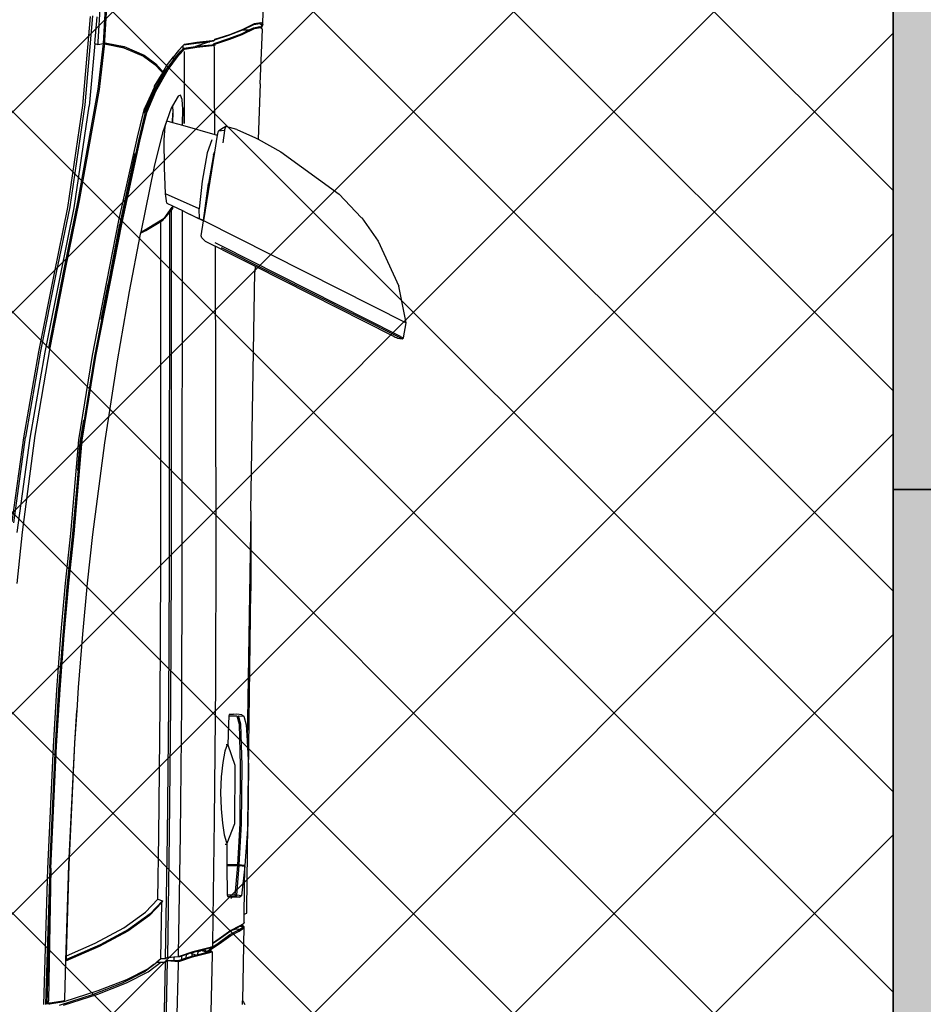
# Model space of a CAD drawing. Units: inches. Extents: x 2167 to 2589, y 1680 to 2489.
# Tile 19 of 38: x 2387 to 2419, y 1761 to 1796. Entities that reach past the tile are written whole.
import ezdxf

# ---------------------------------------------------------------- set-up
doc = ezdxf.new("R2010")
doc.units = ezdxf.units.IN
doc.header["$MEASUREMENT"] = 0
doc.layers.get('0').update_dxf_attribs({"color": 250})
doc.layers.add('A-FLOR-PATT', color=254, linetype='Continuous', lineweight=13, true_color=0xfeeab9)
for name, color, linetype, lineweight in [('A-WALL-PATT', 250, 'Continuous', 13), ('C-PRKG-VEHS', 8, 'Continuous', 13), ('L-PVMT-PATT', 252, 'Continuous', 13), ('walls', 7, 'Continuous', 35)]:
    doc.layers.add(name, color=color, linetype=linetype, lineweight=lineweight)
doc.layers.add('Edges', color=250, linetype='Continuous')

# ---------------------------------------------------------------- blocks, each defined once
blk = doc.blocks.new('Nissan Qashqai pl')
at = {"layer": 'Edges'}
for p, q in [((8.8918, 12.7444), (9.0186, 12.9956)), ((9.0386, 12.9907), (8.9254, 12.7664)), ((9.0186, 12.9956), (8.9731, 12.9865)), ((9.0374, 12.9925), (9.0186, 12.9956)), ((9.0356, 12.9888), (9.0333, 12.9845)), ((9.0356, 12.9888), (9.0374, 12.9925)), ((9.0386, 12.9907), (9.0374, 12.9925)), ((9.0376, 12.985), (9.0386, 12.9907)), ((8.9173, 12.961), (8.9731, 12.9865)), ((9.0333, 12.9845), (8.9232, 12.7662)), ((8.9483, 12.8082), (9.0343, 12.9785)), ((9.0343, 12.9785), (9.0347, 12.9794)), ((9.0347, 12.9794), (9.0362, 12.9822)), ((9.0362, 12.9822), (9.037, 12.9838)), ((9.0371, 12.9841), (9.037, 12.9838)), ((9.0371, 12.9841), (9.0376, 12.985)), ((9.0376, 12.985), (9.0371, 12.9847)), ((8.8885, 12.9405), (8.9173, 12.961)), ((8.8591, 12.9127), (8.8879, 12.94)), ((8.8885, 12.9405), (8.8879, 12.94)), ((8.8066, 12.84), (8.8591, 12.9127)), ((8.7908, 12.812), (8.8066, 12.84)), ((8.6489, 12.8179), (8.5719, 12.8193)), ((8.646, 12.8153), (8.6489, 12.8179)), ((8.6489, 12.8179), (8.6527, 12.8156)), ((8.6547, 12.8176), (8.6537, 12.8167)), ((8.7222, 12.8144), (8.6547, 12.8176)), ((8.646, 12.8153), (8.646, 12.8153)), ((8.6472, 12.8076), (8.646, 12.8153)), ((8.647, 12.8142), (8.6498, 12.8168)), ((8.6482, 12.8067), (8.647, 12.8142)), ((8.6546, 12.7926), (8.6472, 12.8076)), ((8.655, 12.7929), (8.6482, 12.8067)), ((8.6498, 12.8168), (8.6524, 12.8153)), ((8.651, 12.814), (8.652, 12.815)), ((8.6524, 12.8064), (8.651, 12.814)), ((8.652, 12.815), (8.6524, 12.8153)), ((8.6534, 12.8073), (8.652, 12.815)), ((8.6524, 12.8153), (8.6527, 12.8156)), ((8.655, 12.801), (8.6524, 12.8064)), ((8.6527, 12.8156), (8.6537, 12.8167)), ((8.6608, 12.7921), (8.6534, 12.8073)), ((8.6537, 12.8167), (8.6537, 12.8166)), ((8.7222, 12.8144), (8.7908, 12.812)), ((8.7785, 12.7855), (8.7891, 12.8089)), ((8.7891, 12.8089), (8.7908, 12.812)), ((8.928, 12.7679), (8.9483, 12.8082)), ((8.9483, 12.8082), (8.9552, 12.8081)), ((9.2517, 12.8031), (8.9552, 12.8081)), ((8.6606, 12.7768), (8.6546, 12.7926)), ((8.6598, 12.7913), (8.655, 12.801)), ((8.655, 12.7929), (8.655, 12.801)), ((8.6556, 12.7918), (8.655, 12.7929)), ((8.655, 12.7922), (8.655, 12.7929)), ((9.2517, 12.8031), (9.351, 12.803)), ((9.2517, 12.8031), (9.5372, 12.7983)), ((9.641, 12.7991), (9.351, 12.803)), ((9.5052, 12.7918), (9.5069, 12.7941)), ((9.5061, 12.7878), (9.5069, 12.7941)), ((9.5069, 12.7941), (9.5176, 12.7972)), ((9.5176, 12.7972), (9.5372, 12.7983)), ((9.5372, 12.7983), (9.5689, 12.7999)), ((9.5689, 12.7999), (9.641, 12.7991)), ((9.641, 12.7991), (9.6921, 12.7956)), ((9.7466, 12.7978), (9.641, 12.7991)), ((9.692, 12.7943), (9.6913, 12.7886)), ((9.6921, 12.7956), (9.692, 12.7943)), ((9.6922, 12.7943), (9.692, 12.7943)), ((9.6922, 12.7943), (9.6921, 12.7956)), ((9.7526, 12.7946), (9.6921, 12.7956)), ((9.6922, 12.7885), (9.693, 12.7955)), ((9.6922, 12.7885), (9.6922, 12.7943)), ((9.693, 12.7955), (9.7296, 12.7914)), ((9.7511, 12.7979), (9.7466, 12.7978)), ((9.7526, 12.7946), (9.7511, 12.7979)), ((9.7623, 12.7945), (9.7526, 12.7946)), ((9.7623, 12.7945), (9.7643, 12.7937)), ((9.7643, 12.7937), (9.7652, 12.7927)), ((9.7643, 12.7937), (9.7648, 12.7929)), ((9.7648, 12.7929), (9.7648, 12.7929)), ((9.7648, 12.7929), (9.7664, 12.7902)), ((9.7652, 12.7927), (9.7665, 12.7907)), ((9.7667, 12.7933), (9.7665, 12.7907)), ((9.7677, 12.7944), (9.7667, 12.7933)), ((9.7676, 12.7931), (9.7667, 12.7933)), ((9.7673, 12.7899), (9.7676, 12.7931)), ((9.769, 12.7926), (9.7676, 12.7931)), ((9.7677, 12.7944), (9.7677, 12.7944)), ((9.77, 12.7936), (9.7677, 12.7944)), ((9.7677, 12.7944), (9.8598, 12.7928)), ((9.7712, 12.7892), (9.769, 12.7926)), ((9.7734, 12.7884), (9.77, 12.7936)), ((9.8598, 12.7928), (9.8614, 12.7937)), ((9.8643, 12.7927), (9.8598, 12.7928)), ((9.8614, 12.7937), (9.8647, 12.7956)), ((8.6616, 12.7758), (8.6556, 12.7918)), ((8.6657, 12.7758), (8.6598, 12.7913)), ((8.6667, 12.7767), (8.6608, 12.7921)), ((8.7785, 12.7855), (8.7751, 12.7719)), ((9.5037, 12.7806), (9.5045, 12.7814)), ((9.5052, 12.7918), (9.5044, 12.7856)), ((9.5044, 12.7856), (9.5045, 12.7814)), ((9.5045, 12.7814), (9.5045, 12.7759)), ((9.5168, 12.7904), (9.5061, 12.7878)), ((9.5061, 12.7856), (9.5167, 12.7883)), ((9.5063, 12.7755), (9.5061, 12.7856)), ((9.5167, 12.7883), (9.5679, 12.7899)), ((9.5679, 12.792), (9.5168, 12.7904)), ((9.5678, 12.7837), (9.5426, 12.7747)), ((9.64, 12.7831), (9.5678, 12.7837)), ((9.6401, 12.7914), (9.5679, 12.792)), ((9.5679, 12.7899), (9.64, 12.7892)), ((9.64, 12.7892), (9.6912, 12.7865)), ((9.6645, 12.7737), (9.64, 12.7831)), ((9.6913, 12.7886), (9.6401, 12.7914)), ((9.6912, 12.7811), (9.6911, 12.7796)), ((9.6913, 12.7886), (9.6912, 12.7865)), ((9.6912, 12.7865), (9.6912, 12.7811)), ((9.692, 12.7811), (9.6912, 12.7811)), ((9.692, 12.7811), (9.6921, 12.7864)), ((9.692, 12.7796), (9.692, 12.7811)), ((9.6922, 12.7885), (9.6921, 12.7864)), ((9.6921, 12.7864), (9.7288, 12.7832)), ((9.7288, 12.7854), (9.6922, 12.7885)), ((9.7288, 12.7832), (9.7287, 12.7734)), ((9.7296, 12.7914), (9.7288, 12.7854)), ((9.7306, 12.7834), (9.7288, 12.7854)), ((9.7288, 12.7854), (9.7288, 12.7832)), ((9.7288, 12.7832), (9.7306, 12.7834)), ((9.7296, 12.7914), (9.7314, 12.7895)), ((9.7305, 12.7738), (9.7306, 12.7834)), ((9.7306, 12.7834), (9.7314, 12.7895)), ((9.7314, 12.7895), (9.7313, 12.7798)), ((9.7665, 12.7904), (9.7664, 12.7902)), ((9.7664, 12.7902), (9.7674, 12.7885)), ((9.7665, 12.7907), (9.7676, 12.7889)), ((9.7673, 12.7897), (9.7673, 12.7899)), ((9.7673, 12.7897), (9.7676, 12.7889)), ((9.7674, 12.7885), (9.7728, 12.7781)), ((9.7676, 12.7889), (9.7684, 12.7875)), ((9.7676, 12.7887), (9.7678, 12.7882)), ((9.7684, 12.7875), (9.7717, 12.781)), ((9.7707, 12.7848), (9.7709, 12.7893)), ((9.7717, 12.781), (9.7707, 12.7848)), ((9.7709, 12.7893), (9.7712, 12.7892)), ((9.7724, 12.7874), (9.7712, 12.7892)), ((9.7717, 12.781), (9.7738, 12.7771)), ((9.7778, 12.777), (9.7724, 12.7874)), ((9.7788, 12.778), (9.7734, 12.7884)), ((8.6667, 12.7584), (8.6606, 12.7768)), ((8.6675, 12.758), (8.6616, 12.7758)), ((8.6718, 12.7574), (8.6657, 12.7758)), ((8.6728, 12.7584), (8.6667, 12.7767)), ((8.7751, 12.7719), (8.7779, 12.7668)), ((8.7798, 12.7703), (8.7751, 12.7719)), ((8.7798, 12.7703), (8.7807, 12.763)), ((8.7798, 12.7703), (8.7954, 12.7683)), ((9.5045, 12.7759), (9.5063, 12.7755)), ((9.5063, 12.7755), (9.5168, 12.7751)), ((9.5168, 12.7751), (9.5423, 12.7746)), ((9.5423, 12.7746), (9.5422, 12.7736)), ((9.5422, 12.7736), (9.5422, 12.7725)), ((9.5422, 12.7736), (9.5424, 12.7735)), ((9.5426, 12.7747), (9.5423, 12.7746)), ((9.5426, 12.7747), (9.5424, 12.7735)), ((9.5424, 12.7735), (9.5503, 12.7706)), ((9.5503, 12.7706), (9.5641, 12.7681)), ((9.6395, 12.7676), (9.654, 12.7697)), ((9.654, 12.7697), (9.6633, 12.7726)), ((9.6633, 12.7726), (9.6645, 12.7737)), ((9.6655, 12.7733), (9.6645, 12.7737)), ((9.6655, 12.7733), (9.6911, 12.7732)), ((9.6655, 12.7713), (9.6655, 12.7733)), ((9.6911, 12.7796), (9.6911, 12.7732)), ((9.6911, 12.7732), (9.692, 12.7733)), ((9.692, 12.7733), (9.692, 12.7796)), ((9.692, 12.7733), (9.7287, 12.7734)), ((9.7287, 12.7734), (9.7305, 12.7738)), ((9.7305, 12.7738), (9.7313, 12.7798)), ((9.733, 12.7782), (9.7313, 12.7798)), ((9.7728, 12.7781), (9.7832, 12.7637)), ((9.7738, 12.7771), (9.7842, 12.7627)), ((9.7883, 12.7626), (9.7778, 12.777)), ((9.7894, 12.7636), (9.7788, 12.778)), ((8.6675, 12.758), (8.6667, 12.7584)), ((8.6679, 12.7578), (8.6675, 12.758)), ((8.6676, 12.7576), (8.6675, 12.7576)), ((8.6675, 12.7576), (8.6675, 12.7576)), ((8.6675, 12.7576), (8.6676, 12.7576)), ((8.6676, 12.7576), (8.6677, 12.7576)), ((8.6677, 12.7576), (8.6677, 12.7576)), ((8.6677, 12.7576), (8.6682, 12.7576)), ((8.6682, 12.7576), (8.6679, 12.7578)), ((8.6682, 12.7576), (8.6692, 12.7566)), ((8.6682, 12.7572), (8.6682, 12.7576)), ((8.6684, 12.7554), (8.6682, 12.7572)), ((8.6682, 12.7572), (8.6692, 12.7566)), ((8.6692, 12.7566), (8.6697, 12.7519)), ((8.6729, 12.7568), (8.6718, 12.7574)), ((8.674, 12.7578), (8.6728, 12.7584)), ((8.6733, 12.7566), (8.6729, 12.7568)), ((8.6735, 12.7544), (8.6733, 12.7566)), ((8.6742, 12.7576), (8.674, 12.7578)), ((8.6742, 12.7584), (8.6743, 12.7582)), ((8.6744, 12.755), (8.6742, 12.7576)), ((8.6744, 12.7576), (8.6742, 12.7576)), ((8.6744, 12.7578), (8.6744, 12.7576)), ((8.6773, 12.7577), (8.6744, 12.7576)), ((8.6791, 12.7578), (8.677, 12.7578)), ((8.6791, 12.7577), (8.6773, 12.7577)), ((8.7205, 12.7579), (8.6791, 12.7578)), ((8.6791, 12.7577), (8.6791, 12.7578)), ((8.6878, 12.7577), (8.6791, 12.7578)), ((8.6878, 12.7577), (8.6791, 12.7577)), ((8.6878, 12.7577), (8.6878, 12.7577)), ((8.6911, 12.7577), (8.6878, 12.7577)), ((8.7205, 12.7579), (8.6911, 12.7577)), ((8.7849, 12.7582), (8.7205, 12.7579)), ((8.7734, 12.7181), (8.7849, 12.7582)), ((8.7779, 12.7668), (8.7807, 12.763)), ((8.7849, 12.7615), (8.7807, 12.763)), ((8.7849, 12.7615), (8.7858, 12.7613)), ((8.7849, 12.7582), (8.7856, 12.7608)), ((8.7858, 12.7613), (8.7856, 12.7608)), ((8.7858, 12.7613), (8.807, 12.758)), ((8.8102, 12.7568), (8.807, 12.758)), ((8.807, 12.758), (8.8918, 12.7444)), ((8.8102, 12.7568), (8.8455, 12.7506)), ((8.9171, 12.7464), (8.9233, 12.7586)), ((8.9232, 12.7662), (8.9194, 12.7588)), ((8.925, 12.762), (8.9233, 12.7586)), ((8.9233, 12.7586), (9.2886, 12.7594)), ((8.928, 12.7679), (8.925, 12.762)), ((9.2886, 12.7594), (9.4673, 12.7589)), ((9.4673, 12.7589), (9.6358, 12.7575)), ((9.5641, 12.7681), (9.5818, 12.766)), ((9.5818, 12.766), (9.6016, 12.7651)), ((9.6016, 12.7651), (9.6215, 12.766)), ((9.6215, 12.766), (9.6395, 12.7676)), ((9.6358, 12.7575), (9.7887, 12.7552)), ((9.7832, 12.7637), (9.7887, 12.7552)), ((9.7842, 12.7627), (9.7891, 12.7552)), ((9.7933, 12.7549), (9.7883, 12.7626)), ((9.7965, 12.7526), (9.7894, 12.7636)), ((8.6684, 12.7554), (8.6685, 12.7549)), ((8.6684, 12.755), (8.6684, 12.7554)), ((8.6703, 12.7361), (8.6684, 12.755)), ((8.6697, 12.7519), (8.6698, 12.7516)), ((8.6714, 12.7353), (8.6697, 12.7519)), ((8.6698, 12.7516), (8.6755, 12.7343)), ((8.6754, 12.7353), (8.6735, 12.7544)), ((8.6764, 12.736), (8.6744, 12.755)), ((8.7917, 12.7547), (8.8075, 12.7486)), ((8.8075, 12.7486), (8.8429, 12.7426)), ((8.8918, 12.7444), (8.8455, 12.7506)), ((8.8815, 12.7228), (8.892, 12.7444)), ((8.892, 12.7444), (8.8908, 12.7421)), ((8.8911, 12.7428), (8.8919, 12.7444)), ((8.8911, 12.7428), (8.8919, 12.7444)), ((8.8919, 12.7444), (8.8911, 12.7428)), ((8.8919, 12.7444), (8.8918, 12.7444)), ((8.892, 12.7444), (8.8919, 12.7444)), ((8.8919, 12.7444), (8.8919, 12.7444)), ((8.8919, 12.7444), (8.8919, 12.7444)), ((8.9106, 12.7413), (8.892, 12.7444)), ((8.892, 12.7444), (8.892, 12.7444)), ((8.9171, 12.7464), (8.9131, 12.7421)), ((8.9171, 12.7464), (8.917, 12.7468)), ((9.7887, 12.7552), (9.7891, 12.7552)), ((9.7891, 12.7552), (9.79, 12.7552)), ((9.79, 12.7552), (9.7931, 12.7552)), ((9.7931, 12.7552), (9.7934, 12.7535)), ((9.7931, 12.7552), (9.7933, 12.7549)), ((9.7933, 12.7549), (9.7941, 12.7541)), ((9.7934, 12.7535), (9.7938, 12.7538)), ((9.7934, 12.7535), (9.7937, 12.7524)), ((9.7937, 12.7524), (9.7992, 12.7308)), ((9.7941, 12.7541), (9.7943, 12.7535)), ((9.7955, 12.7516), (9.7943, 12.7535)), ((9.7943, 12.7535), (9.7964, 12.7453)), ((9.7963, 12.7523), (9.7955, 12.7516)), ((9.7963, 12.7523), (9.7963, 12.7524)), ((9.7964, 12.7524), (9.7963, 12.7523)), ((9.7992, 12.7476), (9.7963, 12.7523)), ((9.7967, 12.7526), (9.7964, 12.7524)), ((9.7964, 12.7525), (9.7964, 12.7524)), ((9.7964, 12.7524), (9.7996, 12.7475)), ((9.7964, 12.7453), (9.7992, 12.7476)), ((9.7964, 12.7453), (9.7973, 12.7418)), ((9.7983, 12.7541), (9.7965, 12.7526)), ((9.7965, 12.7526), (9.7967, 12.7526)), ((9.7977, 12.7535), (9.7967, 12.7526)), ((9.7967, 12.7526), (9.7986, 12.7526)), ((9.7982, 12.754), (9.7977, 12.7535)), ((9.7977, 12.7444), (9.7985, 12.7451)), ((9.7985, 12.7451), (9.7977, 12.7431)), ((9.7977, 12.7431), (9.7977, 12.7444)), ((9.7983, 12.7541), (9.7982, 12.754)), ((9.7986, 12.7526), (9.7982, 12.754)), ((9.7986, 12.7544), (9.7983, 12.7541)), ((9.7989, 12.7461), (9.7985, 12.7451)), ((9.7993, 12.755), (9.7986, 12.7544)), ((9.7988, 12.7516), (9.7986, 12.7526)), ((9.7998, 12.7477), (9.7988, 12.7516)), ((9.7998, 12.7466), (9.7989, 12.7461)), ((9.7998, 12.7466), (9.7992, 12.7476)), ((9.7999, 12.7522), (9.7993, 12.755)), ((9.7993, 12.755), (9.8024, 12.7549)), ((9.7996, 12.7475), (9.7998, 12.7477)), ((9.8002, 12.7461), (9.7996, 12.7475)), ((9.8001, 12.7468), (9.7996, 12.7475)), ((9.8001, 12.7468), (9.7998, 12.7477)), ((9.8003, 12.7458), (9.7998, 12.7466)), ((9.8054, 12.7307), (9.7999, 12.7522)), ((9.8002, 12.7461), (9.8001, 12.7468)), ((9.8003, 12.7458), (9.8002, 12.7461)), ((9.8027, 12.7364), (9.8003, 12.7458)), ((9.8024, 12.7549), (9.9426, 12.7518)), ((8.6727, 12.7207), (8.6703, 12.7361)), ((8.6737, 12.7197), (8.6714, 12.7353)), ((8.6755, 12.7343), (8.6754, 12.7353)), ((8.6777, 12.7196), (8.6755, 12.7343)), ((8.6764, 12.7359), (8.6764, 12.736)), ((8.6788, 12.7205), (8.6764, 12.7359)), ((8.8429, 12.7426), (8.8771, 12.7388)), ((8.8771, 12.7388), (8.8585, 12.6969)), ((8.8895, 12.7393), (8.8771, 12.7388)), ((8.8815, 12.7228), (8.8895, 12.7393)), ((8.8908, 12.7421), (8.8895, 12.7393)), ((8.8906, 12.7418), (8.8895, 12.7393)), ((8.8906, 12.7418), (8.8911, 12.7428)), ((8.9131, 12.7421), (8.9106, 12.7413)), ((9.7977, 12.7431), (9.7973, 12.7418)), ((9.7973, 12.7418), (9.7977, 12.7409)), ((9.7973, 12.7418), (9.7977, 12.7399)), ((9.7977, 12.7399), (9.7977, 12.7409)), ((9.7977, 12.7409), (9.7987, 12.7388)), ((9.7977, 12.7399), (9.7978, 12.7397)), ((9.7987, 12.7388), (9.7978, 12.7397)), ((9.7978, 12.7397), (9.7987, 12.7362)), ((9.7987, 12.7388), (9.7992, 12.7377)), ((9.7987, 12.7362), (9.7992, 12.7377)), ((9.7987, 12.7362), (9.8002, 12.7301)), ((9.7992, 12.7377), (9.8027, 12.7364)), ((9.8014, 12.7303), (9.8031, 12.7349)), ((9.8031, 12.7349), (9.8027, 12.7364)), ((9.8043, 12.7303), (9.8031, 12.7349)), ((8.6737, 12.7197), (8.6727, 12.7207)), ((8.6746, 12.7189), (8.6737, 12.7197)), ((8.6785, 12.7189), (8.6777, 12.7196)), ((8.687, 12.7132), (8.6788, 12.7205)), ((8.6818, 12.7204), (8.7012, 12.7203)), ((8.7012, 12.7203), (8.7012, 12.7203)), ((8.7012, 12.7203), (8.7026, 12.7203)), ((8.7026, 12.7203), (8.7026, 12.7203)), ((8.7026, 12.7203), (8.7072, 12.7203)), ((8.7072, 12.7203), (8.7072, 12.7203)), ((8.7072, 12.7203), (8.7273, 12.7202)), ((8.7273, 12.7202), (8.7273, 12.7201)), ((8.7273, 12.7202), (8.7354, 12.7202)), ((8.7354, 12.7201), (8.7354, 12.7202)), ((8.7354, 12.7202), (8.742, 12.7202)), ((8.742, 12.7201), (8.742, 12.7202)), ((8.742, 12.7202), (8.742, 12.7201)), ((8.742, 12.7202), (8.742, 12.7202)), ((8.742, 12.7202), (8.7426, 12.7202)), ((8.7426, 12.7201), (8.7426, 12.7202)), ((8.7426, 12.7202), (8.7433, 12.7202)), ((8.7433, 12.7201), (8.7433, 12.7202)), ((8.7433, 12.7202), (8.7711, 12.7201)), ((8.7711, 12.7201), (8.7516, 12.72)), ((8.8793, 12.7181), (8.8815, 12.7228)), ((9.7992, 12.7308), (9.8044, 12.7151)), ((9.8002, 12.7301), (9.8008, 12.7285)), ((9.8008, 12.7285), (9.8014, 12.7303)), ((9.8008, 12.7285), (9.8014, 12.7265)), ((9.8043, 12.7303), (9.8014, 12.7303)), ((9.8014, 12.7265), (9.803, 12.723)), ((9.8014, 12.7265), (9.8026, 12.723)), ((9.803, 12.723), (9.8026, 12.723)), ((9.8026, 12.723), (9.8046, 12.7171)), ((9.8067, 12.7229), (9.803, 12.723)), ((9.8044, 12.73), (9.8043, 12.7303)), ((9.8067, 12.7229), (9.8044, 12.73)), ((9.8106, 12.715), (9.8054, 12.7307)), ((9.8086, 12.7171), (9.8067, 12.7229)), ((8.6785, 12.7189), (8.6746, 12.7189)), ((8.6805, 12.7132), (8.6746, 12.7189)), ((8.6815, 12.7162), (8.6785, 12.7189)), ((8.6805, 12.7132), (8.6884, 12.7071)), ((8.6815, 12.7162), (8.6818, 12.7154)), ((8.6817, 12.716), (8.6815, 12.7162)), ((8.6817, 12.716), (8.6818, 12.7154)), ((8.6859, 12.7122), (8.6817, 12.716)), ((8.6818, 12.7154), (8.6902, 12.7081)), ((8.6927, 12.7071), (8.6859, 12.7122)), ((8.7042, 12.7002), (8.687, 12.7132)), ((8.6917, 12.7071), (8.6884, 12.7071)), ((8.698, 12.6996), (8.6884, 12.7071)), ((8.6902, 12.7081), (8.6917, 12.7071)), ((8.6917, 12.7071), (8.7075, 12.6955)), ((8.6927, 12.7071), (8.6923, 12.7071)), ((8.7032, 12.6992), (8.6927, 12.7071)), ((8.7415, 12.7177), (8.7361, 12.7158)), ((8.7361, 12.7158), (8.7373, 12.7128)), ((8.7373, 12.7128), (8.7492, 12.7059)), ((8.7534, 12.7185), (8.7415, 12.7177)), ((8.7718, 12.7181), (8.7534, 12.7185)), ((8.7698, 12.7058), (8.7734, 12.7181)), ((8.7734, 12.7181), (8.7718, 12.7181)), ((8.8734, 12.7057), (8.8793, 12.7181)), ((9.3194, 12.7179), (8.8793, 12.7181)), ((9.4919, 12.7173), (9.3194, 12.7179)), ((9.6538, 12.7157), (9.4919, 12.7173)), ((9.802, 12.7133), (9.6538, 12.7157)), ((9.8051, 12.7132), (9.802, 12.7133)), ((9.8044, 12.7151), (9.8051, 12.7132)), ((9.8046, 12.7171), (9.8086, 12.7171)), ((9.8046, 12.7171), (9.8055, 12.7143)), ((9.8061, 12.6994), (9.8051, 12.7132)), ((9.8055, 12.7143), (9.8058, 12.7073)), ((9.8058, 12.7073), (9.8098, 12.7073)), ((9.8058, 12.7073), (9.8061, 12.6994)), ((9.8096, 12.7142), (9.8086, 12.7171)), ((9.8098, 12.7073), (9.8096, 12.7142)), ((9.8101, 12.6993), (9.8098, 12.7073)), ((9.8101, 12.6993), (9.8112, 12.7131)), ((9.8112, 12.7131), (9.8106, 12.715)), ((9.8143, 12.713), (9.8112, 12.7131)), ((9.9414, 12.71), (9.8143, 12.713)), ((8.7071, 12.6942), (8.698, 12.6996)), ((8.7302, 12.684), (8.7032, 12.6992)), ((8.7312, 12.6851), (8.7042, 12.7002)), ((8.7075, 12.6955), (8.7346, 12.6806)), ((8.7492, 12.7059), (8.7572, 12.7062)), ((8.7492, 12.7059), (8.7524, 12.704)), ((8.7524, 12.704), (8.7828, 12.6934)), ((8.7572, 12.7062), (8.7698, 12.7058)), ((8.7698, 12.7057), (8.7583, 12.706)), ((8.7678, 12.6988), (8.7698, 12.7057)), ((8.7748, 12.6967), (8.7678, 12.6988)), ((8.7698, 12.7057), (8.7698, 12.7058)), ((8.7916, 12.6954), (8.7748, 12.6967)), ((8.8259, 12.6959), (8.7916, 12.6954)), ((8.8585, 12.6969), (8.8259, 12.6959)), ((8.87, 12.6987), (8.8585, 12.6969)), ((8.87, 12.6987), (8.8734, 12.7057)), ((8.8734, 12.7057), (8.8768, 12.7057)), ((8.8751, 12.7054), (8.8768, 12.7057)), ((8.8893, 12.6956), (8.8751, 12.7054)), ((8.8768, 12.7057), (8.879, 12.704)), ((8.879, 12.704), (9.3198, 12.7039)), ((8.879, 12.704), (8.881, 12.7023)), ((9.3225, 12.7021), (8.881, 12.7023)), ((8.881, 12.7023), (8.8893, 12.6956)), ((8.8893, 12.6956), (8.9021, 12.6745)), ((8.8913, 12.6936), (8.8893, 12.6956)), ((9.3198, 12.7039), (9.4922, 12.7033)), ((9.4936, 12.7013), (9.3225, 12.7021)), ((9.4922, 12.7033), (9.654, 12.7018)), ((9.6552, 12.6997), (9.4936, 12.7013)), ((9.654, 12.7018), (9.8061, 12.6994)), ((9.8078, 12.6971), (9.6552, 12.6997)), ((9.8061, 12.6994), (9.8078, 12.6971)), ((9.8078, 12.6971), (9.8078, 12.6913)), ((9.8119, 12.697), (9.8101, 12.6993)), ((9.8101, 12.6993), (9.9411, 12.6966)), ((9.9393, 12.6944), (9.8119, 12.697)), ((9.8119, 12.6912), (9.8119, 12.697)), ((8.6864, 12.6706), (8.697, 12.685)), ((8.6875, 12.6698), (8.6979, 12.6839)), ((8.6987, 12.6845), (8.6924, 12.676)), ((8.697, 12.685), (8.7055, 12.6927)), ((8.6979, 12.6839), (8.7062, 12.6915)), ((8.7062, 12.6915), (8.6987, 12.6845)), ((8.7055, 12.6927), (8.7071, 12.6942)), ((8.7062, 12.6915), (8.7067, 12.6919)), ((8.7067, 12.6919), (8.7083, 12.6934)), ((8.7071, 12.6942), (8.7083, 12.6934)), ((8.7083, 12.6934), (8.7083, 12.6934)), ((8.7083, 12.6934), (8.7083, 12.6934)), ((8.7102, 12.6923), (8.7083, 12.6934)), ((8.7083, 12.6934), (8.7083, 12.6934)), ((8.7108, 12.6919), (8.7102, 12.6923)), ((8.7102, 12.6923), (8.7102, 12.6923)), ((8.7257, 12.6833), (8.7108, 12.6919)), ((8.7248, 12.6836), (8.7108, 12.6919)), ((8.7257, 12.6833), (8.7248, 12.6836)), ((8.7257, 12.6832), (8.7257, 12.6833)), ((8.7257, 12.6832), (8.7508, 12.672)), ((8.7529, 12.6741), (8.7302, 12.684)), ((8.7574, 12.6737), (8.7312, 12.6851)), ((8.7828, 12.6934), (8.8245, 12.6828)), ((8.8245, 12.6828), (8.9063, 12.6663)), ((8.8927, 12.6913), (8.8913, 12.6936)), ((9.3224, 12.6911), (8.8927, 12.6913)), ((8.9041, 12.6725), (8.8927, 12.6913)), ((9.3225, 12.6911), (9.3224, 12.6911)), ((9.4936, 12.6904), (9.3225, 12.6911)), ((9.6552, 12.6888), (9.4936, 12.6904)), ((9.7337, 12.6875), (9.6552, 12.6888)), ((9.7337, 12.6875), (9.7357, 12.6935)), ((9.7499, 12.6721), (9.7337, 12.6875)), ((9.7357, 12.6935), (9.7378, 12.6924)), ((9.7357, 12.6935), (9.7519, 12.678)), ((9.7378, 12.6924), (9.754, 12.677)), ((9.8078, 12.6913), (9.7378, 12.6924)), ((9.8078, 12.6913), (9.8119, 12.6862)), ((9.8241, 12.6756), (9.8119, 12.6912)), ((9.8119, 12.6862), (9.8119, 12.6912)), ((9.8147, 12.6826), (9.8119, 12.6862)), ((8.6759, 12.6459), (8.6864, 12.6706)), ((8.6883, 12.6704), (8.6777, 12.6457)), ((8.6924, 12.676), (8.6883, 12.6704)), ((8.6924, 12.676), (8.6924, 12.6762)), ((8.7346, 12.6806), (8.7491, 12.6738)), ((8.7346, 12.6806), (8.7577, 12.6709)), ((8.7508, 12.672), (8.7491, 12.6738)), ((8.7491, 12.6738), (8.7576, 12.6699)), ((8.7532, 12.6708), (8.7508, 12.672)), ((8.7529, 12.6741), (8.7577, 12.6709)), ((8.757, 12.6724), (8.7529, 12.6741)), ((8.7575, 12.6698), (8.7532, 12.6708)), ((8.7587, 12.672), (8.757, 12.6724)), ((8.7931, 12.6653), (8.7574, 12.6737)), ((8.7582, 12.6707), (8.7576, 12.6699)), ((8.7577, 12.6709), (8.7582, 12.6707)), ((8.759, 12.6717), (8.7582, 12.6707)), ((8.7587, 12.672), (8.759, 12.6717)), ((8.7591, 12.6719), (8.7587, 12.672)), ((8.7591, 12.6719), (8.759, 12.6717)), ((8.7925, 12.664), (8.7591, 12.6719)), ((8.9021, 12.6745), (8.9063, 12.6663)), ((8.9075, 12.6661), (8.9041, 12.6725)), ((9.7692, 12.6453), (9.7499, 12.6721)), ((9.7519, 12.678), (9.7713, 12.6512)), ((9.754, 12.677), (9.7733, 12.6502)), ((9.8147, 12.6826), (9.8147, 12.6826)), ((9.8147, 12.6826), (9.8201, 12.6756)), ((9.8241, 12.6706), (9.8147, 12.6826)), ((9.8201, 12.6756), (9.8338, 12.6486)), ((9.8378, 12.6485), (9.8241, 12.6756)), ((9.8378, 12.6435), (9.8241, 12.6706)), ((8.6772, 12.6454), (8.6875, 12.6698)), ((8.7576, 12.6699), (8.7575, 12.6698)), ((8.7881, 12.6621), (8.7575, 12.6698)), ((8.8918, 12.6392), (8.7881, 12.6621)), ((8.8941, 12.6418), (8.7925, 12.664)), ((8.8942, 12.6432), (8.7931, 12.6653)), ((8.8083, 12.6591), (8.8954, 12.6403)), ((8.9063, 12.6663), (8.9075, 12.6661)), ((8.9075, 12.6661), (8.9087, 12.6658)), ((8.9087, 12.6658), (8.9797, 12.6518)), ((8.9797, 12.6518), (9.0656, 12.6372)), ((9.7713, 12.6512), (9.7905, 12.6158)), ((9.7733, 12.6502), (9.7925, 12.6148)), ((9.8338, 12.6486), (9.8475, 12.613)), ((9.8516, 12.6129), (9.8378, 12.6485)), ((8.6716, 12.6242), (8.6759, 12.6459)), ((8.6772, 12.6454), (8.6721, 12.6201)), ((8.6777, 12.6457), (8.6727, 12.6213)), ((8.9679, 12.6241), (8.8918, 12.6392)), ((9.0601, 12.6092), (8.8941, 12.6418)), ((8.9696, 12.6285), (8.8942, 12.6432)), ((8.8961, 12.6401), (8.9704, 12.6257)), ((9.0656, 12.6372), (9.1676, 12.6212)), ((9.7885, 12.6099), (9.7692, 12.6453)), ((9.8516, 12.6079), (9.8378, 12.6435)), ((8.6197, 12.6241), (8.6683, 12.6215)), ((8.6721, 12.6201), (8.6204, 12.6229)), ((8.6683, 12.6215), (8.671, 12.6214)), ((8.671, 12.6214), (8.6716, 12.6242)), ((9.0591, 12.6065), (8.9679, 12.6241)), ((9.06, 12.6106), (8.9696, 12.6285)), ((8.9704, 12.6257), (8.9708, 12.6256)), ((8.9708, 12.6256), (9.0143, 12.6169)), ((8.622, 12.6161), (8.6699, 12.6132)), ((8.6721, 12.6093), (8.6387, 12.6123)), ((8.6699, 12.6132), (8.6721, 12.613)), ((8.671, 12.6214), (8.6721, 12.6201)), ((8.6727, 12.6213), (8.6721, 12.6201)), ((8.6733, 12.6129), (8.6721, 12.6201)), ((8.7287, 12.6134), (8.6721, 12.6201)), ((8.6721, 12.6127), (8.6721, 12.613)), ((8.6721, 12.613), (8.6733, 12.6129)), ((8.6721, 12.6093), (8.6733, 12.6129)), ((8.6721, 12.6093), (8.7496, 12.6025)), ((8.6727, 12.6213), (8.6753, 12.621)), ((8.6753, 12.621), (8.7292, 12.6146)), ((8.8666, 12.5888), (8.7287, 12.6134)), ((8.7292, 12.6146), (8.8666, 12.5901)), ((9.1644, 12.5938), (9.06, 12.6106)), ((9.1676, 12.6212), (9.2814, 12.6065)), ((9.8039, 12.5741), (9.7885, 12.6099)), ((9.7905, 12.6158), (9.8087, 12.574)), ((9.7925, 12.6148), (9.8107, 12.573)), ((9.8475, 12.613), (9.8611, 12.5708)), ((9.8652, 12.5704), (9.8516, 12.6129)), ((8.6375, 12.6066), (8.7481, 12.5968)), ((8.6386, 12.6037), (8.7491, 12.594)), ((8.8761, 12.5839), (8.7496, 12.6025)), ((9.1639, 12.5895), (9.0591, 12.6065)), ((9.1645, 12.5924), (9.0601, 12.6092)), ((9.2814, 12.6065), (9.3416, 12.5999)), ((9.3416, 12.5999), (9.4048, 12.5941)), ((9.8652, 12.5654), (9.8516, 12.6079)), ((8.7481, 12.5968), (8.8745, 12.5782)), ((8.7491, 12.594), (8.8754, 12.5755)), ((8.8666, 12.5901), (8.9521, 12.5726)), ((8.9522, 12.5713), (8.8666, 12.5888)), ((9.1393, 12.5951), (9.1647, 12.591)), ((9.2801, 12.5794), (9.1639, 12.5895)), ((9.2803, 12.5836), (9.1644, 12.5938)), ((9.2804, 12.5821), (9.1645, 12.5924)), ((9.1647, 12.591), (9.1668, 12.5908)), ((9.1668, 12.5908), (9.2019, 12.5877)), ((9.4048, 12.5941), (9.471, 12.5888)), ((9.471, 12.5888), (9.4997, 12.5869)), ((9.5404, 12.5844), (9.4997, 12.5869)), ((9.4997, 12.5869), (9.5403, 12.5842)), ((8.8745, 12.5782), (8.9583, 12.5609)), ((8.8754, 12.5755), (8.9591, 12.5583)), ((8.9598, 12.5666), (8.8761, 12.5839)), ((9.3418, 12.5729), (9.2801, 12.5794)), ((9.3418, 12.5771), (9.2803, 12.5836)), ((9.3419, 12.5756), (9.2804, 12.5821)), ((9.4062, 12.5713), (9.3418, 12.5771)), ((9.4064, 12.5671), (9.3418, 12.5729)), ((9.4063, 12.5699), (9.3419, 12.5756)), ((9.5403, 12.5842), (9.6913, 12.5767)), ((9.6912, 12.5774), (9.5404, 12.5844)), ((9.8039, 12.5741), (9.6912, 12.5774)), ((9.6913, 12.5767), (9.8099, 12.573)), ((9.8087, 12.574), (9.8039, 12.5741)), ((9.8099, 12.573), (9.8087, 12.574)), ((9.8099, 12.573), (9.8107, 12.573)), ((9.8107, 12.573), (9.8573, 12.5716)), ((8.9521, 12.5726), (9.0495, 12.5536)), ((9.0497, 12.5523), (8.9522, 12.5713)), ((8.9583, 12.5609), (9.0538, 12.5419)), ((9.0552, 12.5477), (8.9598, 12.5666)), ((9.4735, 12.5663), (9.4062, 12.5713)), ((9.4736, 12.5648), (9.4063, 12.5699)), ((9.4739, 12.5621), (9.4064, 12.5671)), ((9.5437, 12.5619), (9.4735, 12.5663)), ((9.5438, 12.5605), (9.4736, 12.5648)), ((9.5443, 12.5579), (9.4739, 12.5621)), ((9.6953, 12.5549), (9.5437, 12.5619)), ((9.6954, 12.5535), (9.5438, 12.5605)), ((9.8573, 12.5716), (9.8603, 12.5715)), ((9.8603, 12.5715), (9.8605, 12.5696)), ((9.8611, 12.5708), (9.8603, 12.5715)), ((9.8605, 12.5696), (9.8626, 12.5564)), ((9.8612, 12.5707), (9.8611, 12.5708)), ((9.8612, 12.5707), (9.8615, 12.5688)), ((9.8615, 12.5688), (9.8635, 12.5556)), ((8.9591, 12.5583), (9.0546, 12.5394)), ((9.0495, 12.5536), (9.1584, 12.5351)), ((9.696, 12.551), (9.5443, 12.5579)), ((9.6953, 12.5549), (9.8598, 12.5517)), ((9.6953, 12.5549), (9.863, 12.5497)), ((9.6954, 12.5535), (9.8641, 12.5483)), ((9.8644, 12.5459), (9.696, 12.551)), ((9.8629, 12.5516), (9.8598, 12.5517)), ((9.8626, 12.5564), (9.8627, 12.5532)), ((9.8637, 12.5532), (9.8627, 12.5532)), ((9.8627, 12.5532), (9.8629, 12.5516)), ((9.8629, 12.5516), (9.863, 12.5497)), ((9.8641, 12.5483), (9.863, 12.5497)), ((9.8635, 12.5556), (9.8637, 12.5532)), ((9.8643, 12.5532), (9.8637, 12.5532)), ((9.8637, 12.5532), (9.8638, 12.5508)), ((9.8638, 12.5508), (9.8641, 12.5483)), ((9.0538, 12.5419), (9.1605, 12.5233)), ((9.0546, 12.5394), (9.1612, 12.5208)), ((9.1617, 12.5292), (9.0552, 12.5477)), ((9.1584, 12.5351), (9.2783, 12.5191)), ((9.2789, 12.5131), (9.1617, 12.5292)), ((9.2669, 12.5088), (9.1605, 12.5233)), ((9.1612, 12.5208), (9.2656, 12.5065)), ((9.2783, 12.5191), (9.3422, 12.5126))]:
    blk.add_line(p, q, dxfattribs=at)
blk = doc.blocks.new('car')
blk.add_blockref('Nissan Qashqai pl', (-9.7433, -11.9151))
blk = doc.blocks.new('carr')
blk.add_blockref('car', (0.5124, -0.007))

msp = doc.modelspace()

# ---------------------------------------------------------------- hatches: boundary and pattern name
at = {"layer": 'A-FLOR-PATT'}
h = msp.add_hatch(color=256, dxfattribs=at)
h.dxf.hatch_style = 1
h.paths.add_polyline_path([(2525.548, 1864.695), (2455.041, 1864.695), (2455.041, 1855.153), (2455.041, 1830.653), (2525.548, 1830.653)])
h.paths.add_polyline_path([(2455.041, 1855.153), (2452.048, 1855.153), (2452.048, 1864.695), (2426.208, 1864.695), (2422.048, 1864.695), (2422.048, 1788.195), (2467.347, 1788.195), (2467.347, 1812.195), (2452.048, 1812.195), (2452.048, 1830.653), (2455.041, 1830.653)])
h.paths.add_polyline_path([(2419.685, 1779.195), (2417.548, 1779.195), (2417.548, 1696.695), (2419.685, 1696.695)])
at = {"layer": 'A-WALL-PATT'}
h = msp.add_hatch(color=256, dxfattribs=at)
h.dxf.hatch_style = 1
h.paths.add_polyline_path([(2274.738, 1855.042), (2224.048, 1855.042), (2224.048, 2003.119), (2215.048, 2003.119), (2215.048, 1846.042), (2274.738, 1846.042)])
h.paths.add_polyline_path([(2354.886, 1855.042), (2330.895, 1855.042), (2330.895, 1846.042), (2354.773, 1846.042), (2354.773, 1852.042, -0.01877)])
h.paths.add_polyline_path([(2422.048, 1864.695), (2426.208, 1864.695), (2426.208, 1867.924), (2426.208, 1869.195), (2422.048, 1869.195), (2422.048, 1916.243), (2417.548, 1916.243), (2417.548, 1855.042), (2394.773, 1855.042), (2394.773, 1852.042), (2394.773, 1846.042), (2417.548, 1846.042), (2417.548, 1779.195), (2427.738, 1779.195), (2427.738, 1783.941), (2427.738, 1788.195), (2422.048, 1788.195)])
at = {"layer": 'L-PVMT-PATT'}
h = msp.add_hatch(dxfattribs=at)
h.set_pattern_fill('ANSI37', color=256, scale=40)
h.paths.add_polyline_path([(2417.548, 1783.695), (2417.548, 1846.042), (2239.361, 1846.042), (2239.361, 1687.695), (2369.843, 1687.695), (2369.843, 1696.695), (2375.607, 1696.695), (2416.107, 1696.695), (2417.548, 1696.695)])

# ---------------------------------------------------------------- linework, layer by layer
at = {"layer": 'walls'}
for p, q in [((2417.548, 1846.042), (2417.548, 1779.195)), ((2417.548, 1783.695), (2417.548, 1696.695)), ((2427.738, 1779.195), (2417.548, 1779.195))]:
    msp.add_line(p, q, dxfattribs=at)

# ---------------------------------------------------------------- block references
at = {"layer": 'C-PRKG-VEHS', "xscale": 28.42784210623918, "yscale": 28.42784210623918, "zscale": 28.42784210623918, "rotation": 270}
msp.add_blockref('carr', (2369.852, 1779.037), dxfattribs=at)

doc.saveas('drawing.dxf')
